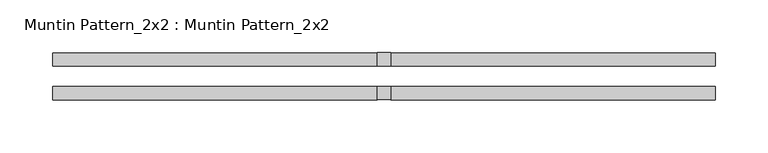
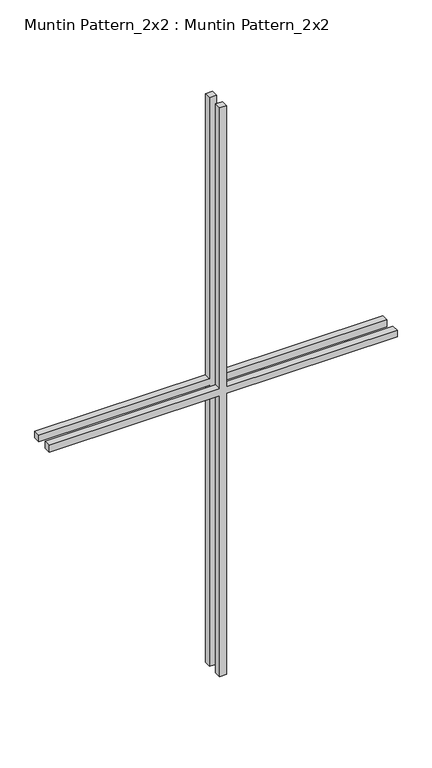
"""IFC4 building model written with IfcOpenShell, lengths in millimetres: proxy geometry, Muntin Pattern_2x2 : Muntin Pattern_2x2."""

from ifc_helpers import new_model, si_unit, frame, origin, place, context, project, spatial, polyline, outline, extrude, source, transform, mapped, element, save


def muntin_pattern_2x2_muntin_pattern_2x2_0a3992d1(model_context):
    return source(origin(), model_context, "Body", "SweptSolid", [
        extrude(outline(polyline([(546.1, -6.35), (546.1, -312.7375), (533.4, -312.7375), (533.4, -6.35), (0.0, -6.35), (0.0, 6.35), (533.4, 6.35), (533.4, 312.7375), (546.1, 312.7375), (546.1, 6.35), (1079.5, 6.35), (1079.5, -6.35), (546.1, -6.35)])), frame((0.0, 9.525, 0.0), z_axis=(0.0, 1.0, 0.0), x_axis=(0.0, 0.0, 1.0)), (0.0, 0.0, 1.0), 12.7),
        extrude(outline(polyline([(546.1, -6.35), (546.1, -312.7375), (533.4, -312.7375), (533.4, -6.35), (0.0, -6.35), (0.0, 6.35), (533.4, 6.35), (533.4, 312.7375), (546.1, 312.7375), (546.1, 6.35), (1079.5, 6.35), (1079.5, -6.35), (546.1, -6.35)])), frame((0.0, -22.225, 0.0), z_axis=(0.0, 1.0, 0.0), x_axis=(0.0, 0.0, 1.0)), (0.0, 0.0, 1.0), 12.7),
    ])


if __name__ == "__main__":
    model = new_model("IFC4")
    model_context = context("Model", 3, world=origin())
    ifc_project = project(units=[si_unit("LENGTHUNIT", "METRE", prefix="MILLI")], contexts=[model_context])
    site = spatial("IfcSite", under=ifc_project)
    building = spatial("IfcBuilding", under=site)
    placement = place(None, origin())
    muntin_pattern_2x2_muntin_pattern_2x2_shape = muntin_pattern_2x2_muntin_pattern_2x2_0a3992d1(model_context)
    element("IfcBuildingElementProxy", 1, Name="Muntin Pattern_2x2 : Muntin Pattern_2x2", ObjectType="Muntin Pattern_2x2 : Muntin Pattern_2x2", at=placement, inside=building, context=model_context, shape_type="MappedRepresentation", body=[
        mapped(muntin_pattern_2x2_muntin_pattern_2x2_shape, transform((0.0, 0.0, 0.0), x_axis=(1.0, 0.0, 0.0), y_axis=(0.0, 1.0, 0.0), z_axis=(0.0, 0.0, 1.0))),
    ])
    save(model, "model.ifc")

# Revit data of these elements
# Type "Muntin Pattern_2x2 : Muntin Pattern_2x2"
#   Width [instance default] = 4' - 0"
#   Thickness = 0' - 0 1/2"
#   Height [instance default] = 4' - 0"
#   Distance = 0' - 0 3/4"
#   Interior Material [instance default] = none
#   Exterior Material [instance default] = none
#   Default Elevation = 0
# Element 1 (IfcBuildingElementProxy, "Muntin Pattern_2x2 : Muntin Pattern_2x2")
#   Width = 2' - 0 5/8"
#   Height = 3' - 6 1/2"
#   Interior Material = Wood - Stained
#   Exterior Material = Clad - White
#   Materials on its faces: "Clad - White", "Wood - Stained"
# Materials
#   "Clad - White": class "Wood", colour RGB 242 242 238, transparency 0, Cost = 0
#   "Wood - Stained": class "Wood", colour RGB 224 178 126, transparency 0, Cost = 0
